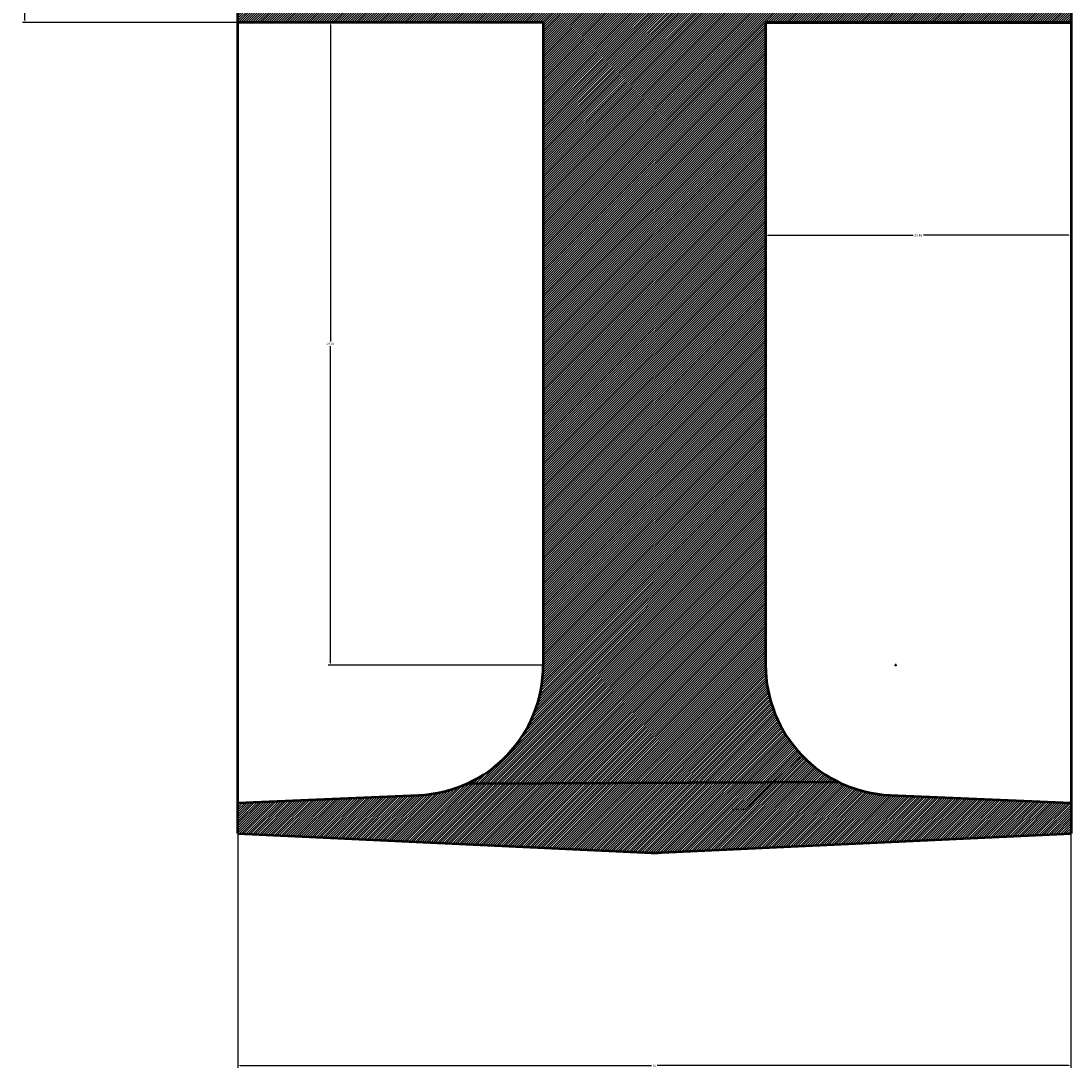
# Model space of a CAD drawing. Units: inches. Extents: x -99 to 284, y -92 to 134.
# Tile 13 of 16: x 187 to 267, y -92 to -11. Entities that reach past the tile are written whole.
import ezdxf

# ---------------------------------------------------------------- set-up
doc = ezdxf.new("R2010")
doc.units = ezdxf.units.IN
doc.header["$MEASUREMENT"] = 0
for name, color, linetype, lineweight in [('M-DIMS', 2, 'Continuous', 18), ('M-HATC', 8, 'Continuous', 18), ('M-OUTL', 7, 'Continuous', 50)]:
    doc.layers.add(name, color=color, linetype=linetype, lineweight=lineweight)
doc.styles.get("Standard").update_dxf_attribs({"font": 'arial.ttf'})
doc.dimstyles.get("Standard").update_dxf_attribs({"dimtxt": 0.18, "dimasz": 0.18, "dimexe": 0.18, "dimexo": 0.0625, "dimgap": 0.09, "dimtad": 0, "dimtih": 1, "dimtoh": 1, "dimdec": 4, "dimzin": 0, "dimdsep": 46, "dimtxsty": 'Standard', "dimcen": 0.09, "dimadec": 0, "dimazin": 0, "dimtfac": 1, "dimtdec": 4, "dimtofl": 0, "dimtmove": 0, "dimatfit": 3, "dimfxl": 1, "dimtolj": 1, "dimtzin": 0, "dimarcsym": 0})

# ---------------------------------------------------------------- blocks, each defined once
blk = doc.blocks.new('*D5')
at = {"layer": 'Defpoints', "color": 0, "transparency": 16777216}
for p in [(203.491, -73.766), (267.491, -73.766), (267.491, -91.61)]:
    blk.add_point(p, dxfattribs=at)
at = {"layer": 'M-DIMS', "color": 0, "lineweight": -2, "transparency": 16777216}
for p, q in [((203.491, -73.828), (203.491, -91.79)), ((267.491, -73.828), (267.491, -91.79)), ((203.671, -91.61), (235.272, -91.61)), ((267.311, -91.61), (235.71, -91.61))]:
    blk.add_line(p, q, dxfattribs=at)
at = {"layer": 'M-DIMS', "color": 0, "transparency": 16777216}
for points in [[(203.671, -91.58), (203.671, -91.64), (203.491, -91.61)], [(267.311, -91.58), (267.311, -91.64), (267.491, -91.61)]]:
    blk.add_solid(points, dxfattribs=at)
at = {"layer": 'M-DIMS', "color": 0, "transparency": 16777216, "insert": (235.491, -91.61), "char_height": 0.18, "attachment_point": 5}
blk.add_mtext('\\A1;64', dxfattribs=at)
blk = doc.blocks.new('*D12')
at = {"layer": 'Defpoints', "color": 0, "transparency": 16777216}
for p in [(187.141, 38.946), (203.491, 38.946), (203.491, -11.467)]:
    blk.add_point(p, dxfattribs=at)
at = {"layer": 'M-DIMS', "color": 0, "lineweight": -2, "transparency": 16777216}
for p, q in [((203.429, 38.946), (186.961, 38.946)), ((187.141, 38.766), (187.141, 13.922)), ((187.141, -11.287), (187.141, 13.558)), ((203.429, -11.467), (186.961, -11.467))]:
    blk.add_line(p, q, dxfattribs=at)
at = {"layer": 'M-DIMS', "color": 0, "transparency": 16777216}
for points in [[(187.111, 38.766), (187.171, 38.766), (187.141, 38.946)], [(187.111, -11.287), (187.171, -11.287), (187.141, -11.467)]]:
    blk.add_solid(points, dxfattribs=at)
at = {"layer": 'M-DIMS', "color": 0, "transparency": 16777216, "insert": (187.141, 13.74), "char_height": 0.18, "attachment_point": 5}
blk.add_mtext('\\A1;50.41', dxfattribs=at)
blk = doc.blocks.new('*D15')
at = {"layer": 'Defpoints', "color": 0, "transparency": 16777216}
for p in [(244.029, -11.467), (267.491, -11.467), (244.029, -27.817)]:
    blk.add_point(p, dxfattribs=at)
at = {"layer": 'M-DIMS', "color": 0, "lineweight": -2, "transparency": 16777216}
for p, q in [((244.029, -11.529), (244.029, -27.997)), ((267.491, -11.529), (267.491, -27.997)), ((244.209, -27.817), (255.365, -27.817)), ((267.311, -27.817), (256.155, -27.817))]:
    blk.add_line(p, q, dxfattribs=at)
at = {"layer": 'M-DIMS', "color": 0, "transparency": 16777216}
for points in [[(244.209, -27.787), (244.209, -27.847), (244.029, -27.817)], [(267.311, -27.787), (267.311, -27.847), (267.491, -27.817)]]:
    blk.add_solid(points, dxfattribs=at)
at = {"layer": 'M-DIMS', "color": 0, "transparency": 16777216, "insert": (255.76, -27.817), "char_height": 0.18, "attachment_point": 5}
blk.add_mtext('\\A1;23.46', dxfattribs=at)
blk = doc.blocks.new('*D18')
at = {"layer": 'Defpoints', "color": 0, "transparency": 16777216}
for p in [(210.603, -11.467), (226.953, -11.467), (226.953, -60.839)]:
    blk.add_point(p, dxfattribs=at)
at = {"layer": 'M-DIMS', "color": 0, "lineweight": -2, "transparency": 16777216}
for p, q in [((226.891, -11.467), (210.423, -11.467)), ((210.603, -11.647), (210.603, -35.971)), ((210.603, -60.659), (210.603, -36.335)), ((226.891, -60.839), (210.423, -60.839))]:
    blk.add_line(p, q, dxfattribs=at)
at = {"layer": 'M-DIMS', "color": 0, "transparency": 16777216}
for points in [[(210.573, -11.647), (210.633, -11.647), (210.603, -11.467)], [(210.573, -60.659), (210.633, -60.659), (210.603, -60.839)]]:
    blk.add_solid(points, dxfattribs=at)
at = {"layer": 'M-DIMS', "color": 0, "transparency": 16777216, "insert": (210.603, -36.153), "char_height": 0.18, "attachment_point": 5}
blk.add_mtext('\\A1;49.37', dxfattribs=at)
blk = doc.blocks.new('*D24')
at = {"layer": 'Defpoints', "color": 0, "transparency": 16777216}
for p in [(254.029, -60.839), (246.806, -67.755)]:
    blk.add_point(p, dxfattribs=at)
at = {"layer": 'M-DIMS', "color": 0, "lineweight": -2, "transparency": 16777216}
for p, q in [((253.939, -60.839), (254.119, -60.839)), ((254.029, -60.929), (254.029, -60.749)), ((242.472, -71.904), (246.676, -67.879)), ((242.292, -71.904), (242.472, -71.904))]:
    blk.add_line(p, q, dxfattribs=at)
at = {"layer": 'M-DIMS', "color": 0, "transparency": 16777216}
blk.add_solid([(246.655, -67.858), (246.697, -67.901), (246.806, -67.755)], dxfattribs=at)
at = {"layer": 'M-DIMS', "color": 0, "transparency": 16777216, "insert": (241.794, -71.904), "char_height": 0.18, "attachment_point": 5}
blk.add_mtext('\\A1;3X R10', dxfattribs=at)

msp = doc.modelspace()

# ---------------------------------------------------------------- hatches: boundary and pattern name
at = {"layer": 'M-HATC'}
h = msp.add_hatch(dxfattribs=at)
h.set_pattern_fill('ANSI31', color=256)
h.set_pattern_definition([(45, (-295.18303, 0), (-0.088388348, 0.088388348), [])])
h.paths.add_polyline_path([(235.9574, 102.7178), (260.4913, 101.5718), (260.4913, 98.6088), (240.4913, 97.7396, -1), (230.4913, 97.7396), (210.4913, 98.6088), (210.4913, 101.573), (235.4326, 102.7424), (235.4913, 102.7396, -0.0233428)])
h.paths.add_polyline_path([(226.9535, 38.946), (203.4913, 38.946), (203.4913, 30.5521), (267.4913, 30.5521), (267.4913, 38.946), (244.0291, 38.946, 0.5614625)])
h.paths.add_polyline_path([(267.4913, 30.5521), (203.4913, 30.5521), (203.4913, 28.5521), (267.4913, 28.5521)])
h.paths.add_polyline_path([(244.0291, -11.4667), (267.4913, -11.4667), (267.4913, -0.9688), (203.4913, -0.9688), (203.4913, -11.4667), (226.9535, -11.4667), (226.9535, -60.8393, -0.294228), (221.0875, -69.9448), (249.6222, -69.8159, -0.2860474), (244.0291, -60.8393)])
h.paths.add_polyline_path([(267.4913, -71.4338), (253.5949, -70.8299, -0.1036016), (249.6222, -69.8159), (221.0875, -69.9448, -0.095981), (217.3877, -70.8299), (203.4913, -71.4338), (203.4913, -73.7656), (235.2571, -75.2549, 0.0117126), (235.4913, -75.2604), (267.4913, -73.7656)])

# ---------------------------------------------------------------- linework, layer by layer
at = {"layer": 'M-OUTL'}
for p, q in [((203.4913, -73.7656), (203.4913, 13.7396)), ((267.4913, 13.7396), (267.4913, -73.7656)), ((226.9535, -11.4667), (203.4913, -11.4667)), ((226.9535, -11.4667), (226.9535, -60.8393)), ((244.0291, -11.4667), (267.4913, -11.4667)), ((267.4913, -11.4667), (244.0291, -11.4667)), ((244.0291, -11.4667), (244.0291, -60.8393)), ((221.0875, -69.9448), (249.6222, -69.8159)), ((203.4913, -73.7656), (203.4913, -70.2604)), ((203.4913, -71.4338), (217.3877, -70.8299)), ((253.5949, -70.8299), (267.4913, -71.4338)), ((203.4913, -73.7656), (235.2571, -75.2549)), ((235.4913, -75.2604), (267.4913, -73.7656))]:
    msp.add_line(p, q, dxfattribs=at)
for centre, radius, start, end in [((216.9535, -60.8393), 10, 272.488516, 0), ((254.0291, -60.8393), 10, 180, 267.511484), ((235.4913, -70.2604), 5, 267.315787, 275.348802)]:
    msp.add_arc(centre, radius, start, end, dxfattribs=at)

# ---------------------------------------------------------------- dimensions: what is measured, and where the dimension line sits
at = {"layer": 'M-DIMS'}
for base, p1, p2, angle, picture, middle in [((187.1413, 38.946), (203.4913, -11.4667), (203.4913, 38.946), 90, '*D12', (187.1413, 13.7396)), ((210.6035, -11.4667), (226.9535, -60.8393), (226.9535, -11.4667), 90, '*D18', (210.6035, -36.153)), ((244.0291, -27.8167), (267.4913, -11.4667), (244.0291, -11.4667), 180, '*D15', (255.7602, -27.8167))]:
    dim = msp.add_linear_dim(base=base, p1=p1, p2=p2, angle=angle, dimstyle='Standard', override={"dimdec": 2, "dimlfac": 1, "dimrnd": 0, "dimzin": 0, "dimdsep": 46, "dimlunit": 2}, dxfattribs=at)
    dim.commit()
    dim.dimension.update_dxf_attribs({"geometry": picture, "text_midpoint": middle})
dim = msp.add_radius_dim(center=(254.0291, -60.8393), mpoint=(246.806, -67.755), text='3X <>', dimstyle='Standard', override={"dimdec": 0, "dimlfac": 1, "dimrnd": 0, "dimzin": 0, "dimdsep": 46, "dimlunit": 2}, dxfattribs=at)
dim.commit()
dim.dimension.update_dxf_attribs({"geometry": '*D24', "text_midpoint": (241.7941, -71.9044), "dimtype": 164})
dim = msp.add_linear_dim(base=(267.4913, -91.6104), p1=(203.4913, -73.7656), p2=(267.4913, -73.7656), dimstyle='Standard', override={"dimdec": 0, "dimlfac": 1, "dimrnd": 0, "dimzin": 0, "dimdsep": 46, "dimlunit": 2}, dxfattribs=at)
dim.commit()
dim.dimension.update_dxf_attribs({"geometry": '*D5', "text_midpoint": (235.4913, -91.6104)})

doc.saveas('drawing.dxf')
